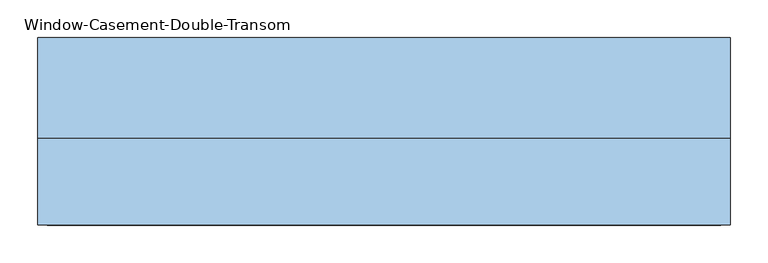
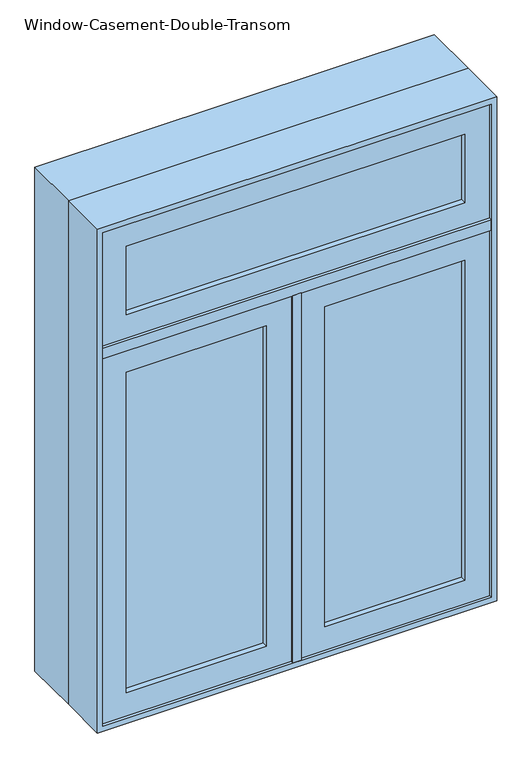
"""IFC4 building model written with IfcOpenShell, lengths in millimetres: window geometry, Window-Casement-Double-Transom."""

from ifc_helpers import new_model, si_unit, frame, origin, place, context, project, spatial, polyline, outline, extrude, faceted_brep, source, transform, mapped, element, save


def window_casement_double_transom_0fae6a54(model_context):
    return source(origin(), model_context, "Body", "SolidModel", [
        faceted_brep([(425.45, -82.55, 2101.85), (-425.45, -82.55, 2101.85), (-425.45, -19.05, 2101.85), (425.45, -19.05, 2101.85), (444.5, -133.35, 2120.9), (-444.5, -133.35, 2120.9), (-444.5, -82.55, 2120.9), (444.5, -82.55, 2120.9), (457.2, -19.05, 2133.6), (-457.2, -19.05, 2133.6), (-457.2, -133.35, 2133.6), (457.2, -133.35, 2133.6), (-425.45, -82.55, 946.15), (-425.45, -19.05, 946.15), (-444.5, -133.35, 927.1), (-444.5, -82.55, 927.1), (-457.2, -19.05, 914.4), (-457.2, -133.35, 914.4), (425.45, -82.55, 946.15), (425.45, -19.05, 946.15), (444.5, -133.35, 927.1), (444.5, -82.55, 927.1), (457.2, -19.05, 914.4), (457.2, -133.35, 914.4)], [[[0, 1, 2, 3]], [[4, 5, 6, 7]], [[8, 9, 10, 11]], [[1, 12, 13, 2]], [[5, 14, 15, 6]], [[9, 16, 17, 10]], [[12, 18, 19, 13]], [[14, 20, 21, 15]], [[16, 22, 23, 17]], [[9, 8, 22, 16], [3, 2, 13, 19]], [[18, 0, 3, 19]], [[7, 6, 15, 21], [1, 0, 18, 12]], [[20, 4, 7, 21]], [[22, 8, 11, 23]], [[11, 10, 17, 23], [5, 4, 20, 14]]]),
        extrude(outline(polyline([(2133.6, -457.2), (914.4, -457.2), (914.4, 457.2), (2133.6, 457.2), (2133.6, -457.2)]), holes=[polyline([(2114.55, 438.15), (933.45, 438.15), (933.45, -438.15), (2114.55, -438.15), (2114.55, 438.15)])]), frame((0.0, -19.05, 0.0), z_axis=(0.0, 1.0, 0.0), x_axis=(0.0, 0.0, 1.0)), (0.0, 0.0, 1.0), 133.35),
        extrude(outline(polyline([(927.1, 9.525), (927.1, 444.5), (1816.1, 444.5), (1816.1, 9.525), (927.1, 9.525)]), holes=[polyline([(984.25, 387.35), (984.25, 66.675), (1758.95, 66.675), (1758.95, 387.35), (984.25, 387.35)])]), frame((0.0, -127.0, 0.0), z_axis=(0.0, 1.0, 0.0), x_axis=(0.0, 0.0, 1.0)), (0.0, 0.0, 1.0), 44.45),
        extrude(outline(polyline([(1816.1, -9.525), (1816.1, -444.5), (927.1, -444.5), (927.1, -9.525), (1816.1, -9.525)]), holes=[polyline([(1758.95, -387.35), (1758.95, -66.675), (984.25, -66.675), (984.25, -387.35), (1758.95, -387.35)])]), frame((0.0, -127.0, 0.0), z_axis=(0.0, 1.0, 0.0), x_axis=(0.0, 0.0, 1.0)), (0.0, 0.0, 1.0), 44.45),
        extrude(outline(polyline([(387.35, -114.3), (66.675, -114.3), (66.675, -107.95), (387.35, -107.95), (387.35, -114.3)])), frame((0.0, 0.0, 984.25), z_axis=(0.0, 0.0, 1.0), x_axis=(1.0, 0.0, 0.0)), (0.0, 0.0, 1.0), 774.7),
        extrude(outline(polyline([(66.675, -95.25), (387.35, -95.25), (387.35, -101.6), (66.675, -101.6), (66.675, -95.25)])), frame((0.0, 0.0, 984.25), z_axis=(0.0, 0.0, 1.0), x_axis=(1.0, 0.0, 0.0)), (0.0, 0.0, 1.0), 774.7),
        extrude(outline(polyline([(-66.675, -114.3), (-387.35, -114.3), (-387.35, -107.95), (-66.675, -107.95), (-66.675, -114.3)])), frame((0.0, 0.0, 984.25), z_axis=(0.0, 0.0, 1.0), x_axis=(1.0, 0.0, 0.0)), (0.0, 0.0, 1.0), 774.7),
        extrude(outline(polyline([(-387.35, -95.25), (-66.675, -95.25), (-66.675, -101.6), (-387.35, -101.6), (-387.35, -95.25)])), frame((0.0, 0.0, 984.25), z_axis=(0.0, 0.0, 1.0), x_axis=(1.0, 0.0, 0.0)), (0.0, 0.0, 1.0), 774.7),
        faceted_brep([(9.525, -133.35, 1816.1), (9.525, -82.55, 1816.1), (30.1625, -82.55, 1816.1), (30.1625, -19.05, 1816.1), (-30.1625, -19.05, 1816.1), (-30.1625, -82.55, 1816.1), (-9.525, -82.55, 1816.1), (-9.525, -133.35, 1816.1), (9.525, -133.35, 927.1), (-9.525, -133.35, 927.1), (-9.525, -82.55, 927.1), (9.525, -82.55, 927.1), (-9.525, -82.55, 946.15), (-30.1625, -82.55, 946.15), (-30.1625, -19.05, 946.15), (30.1625, -19.05, 946.15), (30.1625, -82.55, 946.15), (9.525, -82.55, 946.15)], [[[0, 1, 2, 3, 4, 5, 6, 7]], [[8, 9, 10, 11]], [[7, 9, 8, 0]], [[6, 12, 10, 9, 7]], [[5, 13, 12, 6]], [[4, 14, 13, 5]], [[3, 15, 14, 4]], [[2, 16, 15, 3]], [[1, 17, 16, 2]], [[0, 8, 11, 17, 1]], [[17, 11, 10, 12]], [[12, 13, 14, 15, 16, 17]]]),
        extrude(outline(polyline([(387.35, -114.3), (-387.35, -114.3), (-387.35, -107.95), (387.35, -107.95), (387.35, -114.3)])), frame((0.0, 0.0, 1898.65), z_axis=(0.0, 0.0, 1.0), x_axis=(1.0, 0.0, 0.0)), (0.0, 0.0, 1.0), 165.1),
        extrude(outline(polyline([(-387.35, -95.25), (387.35, -95.25), (387.35, -101.6), (-387.35, -101.6), (-387.35, -95.25)])), frame((0.0, 0.0, 1898.65), z_axis=(0.0, 0.0, 1.0), x_axis=(1.0, 0.0, 0.0)), (0.0, 0.0, 1.0), 165.1),
        extrude(outline(polyline([(444.5, -133.35), (-444.5, -133.35), (-444.5, -82.55), (-425.45, -82.55), (-425.45, -19.05), (425.45, -19.05), (425.45, -82.55), (444.5, -82.55), (444.5, -133.35)])), frame((0.0, 0.0, 1816.1), z_axis=(0.0, 0.0, 1.0), x_axis=(1.0, 0.0, 0.0)), (0.0, 0.0, 1.0), 25.4),
        extrude(outline(polyline([(2120.9, 444.5), (2120.9, -444.5), (1841.5, -444.5), (1841.5, 444.5), (2120.9, 444.5)]), holes=[polyline([(2063.75, -387.35), (2063.75, 387.35), (1898.65, 387.35), (1898.65, -387.35), (2063.75, -387.35)])]), frame((0.0, -127.0, 0.0), z_axis=(0.0, 1.0, 0.0), x_axis=(0.0, 0.0, 1.0)), (0.0, 0.0, 1.0), 44.45),
    ])


if __name__ == "__main__":
    model = new_model("IFC4")
    model_context = context("Model", 3, world=origin())
    ifc_project = project(units=[si_unit("LENGTHUNIT", "METRE", prefix="MILLI")], contexts=[model_context])
    site = spatial("IfcSite", under=ifc_project)
    building = spatial("IfcBuilding", under=site)
    placement = place(None, origin())
    window_casement_double_transom_shape = window_casement_double_transom_0fae6a54(model_context)
    element("IfcWindow", 1, ObjectType="Window-Casement-Double-Transom", at=placement, inside=building, context=model_context, shape_type="MappedRepresentation", body=[
        mapped(window_casement_double_transom_shape, transform((0.0, 0.0, 0.0), x_axis=(1.0, 0.0, 0.0), y_axis=(0.0, 1.0, 0.0), z_axis=(0.0, 0.0, 1.0))),
    ])
    save(model, "model.ifc")

# Revit data of these elements
# Type "Window-Casement-Double-Transom"
#   Type Mark = "23"
#   Fire Rating = "0.5h"
#   Assembly Code = "B2020100"
#   Analytic Construction = "Double glazing - domestic"
#   Window Inset [instance default] = 0' - 0"
#   Wall Thickness [instance default] = 0' - 6"
#   Interior Wall Closure [instance default] = 0' - 2 1/4"
#   Half Width = 1' - 6"
#   Visual Light Transmittance = 0.81
#   Transom Height = 1' - 0"
#   Thermal Resistance (R) = 1.8146 (h·ft²·°F)/BTU
#   Solar Heat Gain Coefficient = 0.76
#   Rough Width = 3' - 0 1/2"
#   Rough Height = 4' - 0 1/2"
#   Open Window Height = 3' - 0"
#   Height = 4' - 0"
#   Heat Transfer Coefficient (U) = 0.5511 BTU/(h·ft²·°F)
#   Frame Extension [instance default] = 0' - 0 1/4"
#   Exterior Wall Closure [instance default] = 0' - 1 1/4"
#   Extension Jamb [instance default] = 0' - 2 1/4"
#   Default Sill Height = 3' - 0"
#   Width = 3' - 0"
#   Muntin Visibility = yes
#   Interior Trim Visibility [instance default] = yes
#   Exterior Trim Visibility [instance default] = yes
#   Extension Jamb Visibility [instance default] = yes
#   Interior Trim Material = Wood - Stained
#   Muntin Pattern = Muntin Pattern_2x2 : Muntin Pattern_2x2
#   Interior Trim = Trim-Window-Interior-Flat : Picture Frame
#   Interior Frame Material = Wood - Stained
#   Glass Panel Material = Glass
#   Exterior Trim Material = Clad - White
#   Exterior Trim = Trim-Window-Exterior-Flat : with Sill
#   Exterior Frame Material = Clad - White
#   Wall Closure = (empty or 0)
# Element 1 (IfcWindow, "Window-Casement-Double-Transom")
#   Wall Thickness = 0' - 9"
#   Extension Jamb = 0' - 5 1/4"
#   Materials on its faces: "Wood - Stained", "Glass", "Clad - White"
# Materials
#   "Wood - Stained": class "Wood", colour RGB 224 178 126, transparency 0, Cost = 0
#   "Glass": class "Glass", colour RGB 0 128 192, transparency 0.75, Description = "Soda Lime Glass", Cost = 0
#   "Clad - White": class "Wood", colour RGB 242 242 238, transparency 0, Cost = 0
